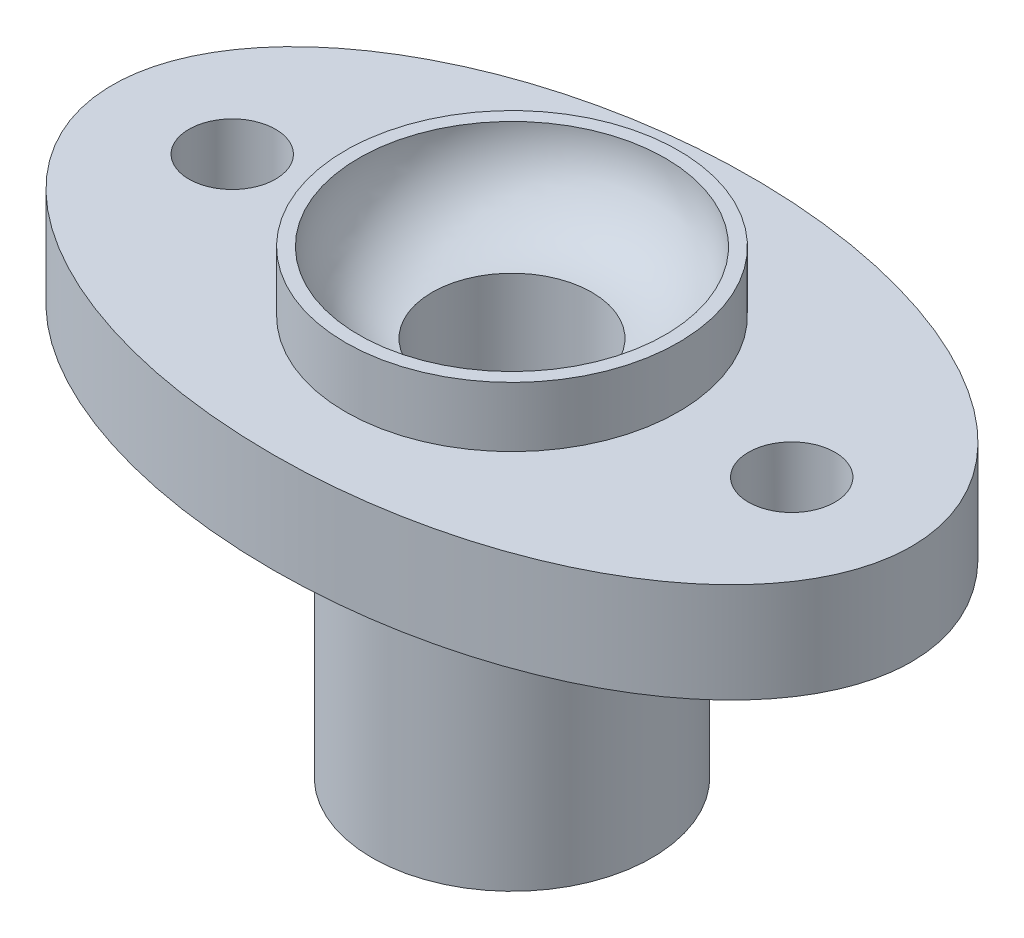
ISO-10303-21;
HEADER;
FILE_DESCRIPTION(('STEP AP214'),'2;1');
FILE_NAME('part.step','',(''),(''),'','','');
FILE_SCHEMA(('AUTOMOTIVE_DESIGN { 1 0 10303 214 1 1 1 1 }'));
ENDSEC;
DATA;
#1=APPLICATION_CONTEXT('core data for automotive mechanical design processes');
#2=APPLICATION_PROTOCOL_DEFINITION('international standard','automotive_design',2000,#1);
#3=PRODUCT_CONTEXT('',#1,'mechanical');
#4=PRODUCT('Part','Part','',(#3));
#5=PRODUCT_RELATED_PRODUCT_CATEGORY('part','',(#4));
#6=PRODUCT_DEFINITION_FORMATION('','',#4);
#7=PRODUCT_DEFINITION_CONTEXT('part definition',#1,'design');
#8=PRODUCT_DEFINITION('design','',#6,#7);
#9=PRODUCT_DEFINITION_SHAPE('','',#8);
#10=(LENGTH_UNIT() NAMED_UNIT(*) SI_UNIT(.MILLI.,.METRE.));
#11=(NAMED_UNIT(*) PLANE_ANGLE_UNIT() SI_UNIT($,.RADIAN.));
#12=(NAMED_UNIT(*) SI_UNIT($,.STERADIAN.) SOLID_ANGLE_UNIT());
#13=UNCERTAINTY_MEASURE_WITH_UNIT(LENGTH_MEASURE(1.E-05),#10,'distance_accuracy_value','');
#14=(GEOMETRIC_REPRESENTATION_CONTEXT(3) GLOBAL_UNCERTAINTY_ASSIGNED_CONTEXT((#13)) GLOBAL_UNIT_ASSIGNED_CONTEXT((#10,
#11,#12)) REPRESENTATION_CONTEXT('',''));
#15=CARTESIAN_POINT('',(0.,0.,0.));
#16=DIRECTION('',(0.,0.,1.));
#17=DIRECTION('',(1.,0.,0.));
#18=AXIS2_PLACEMENT_3D('',#15,#16,#17);
#19=CARTESIAN_POINT('',(0.,-33.9411254969543,0.));
#20=DIRECTION('',(0.,1.,0.));
#21=DIRECTION('',(0.,0.,1.));
#22=AXIS2_PLACEMENT_3D('',#19,#20,#21);
#23=CYLINDRICAL_SURFACE('',#22,12.);
#24=CARTESIAN_POINT('',(0.,2.41154273188011,0.));
#25=DIRECTION('',(0.,1.,0.));
#26=DIRECTION('',(0.,0.,1.));
#27=AXIS2_PLACEMENT_3D('',#24,#25,#26);
#28=CIRCLE('',#27,12.);
#29=CARTESIAN_POINT('',(0.,2.41154273188011,12.));
#30=VERTEX_POINT('',#29);
#31=EDGE_CURVE('E10',#30,#30,#28,.F.);
#32=ORIENTED_EDGE('',*,*,#31,.T.);
#33=EDGE_LOOP('',(#32));
#34=FACE_BOUND('',#33,.T.);
#35=CARTESIAN_POINT('',(0.,57.0417392568986,0.));
#36=DIRECTION('',(0.,1.,0.));
#37=DIRECTION('',(0.,0.,1.));
#38=AXIS2_PLACEMENT_3D('',#35,#36,#37);
#39=CIRCLE('',#38,12.);
#40=CARTESIAN_POINT('',(0.,57.0417392568986,12.));
#41=VERTEX_POINT('',#40);
#42=EDGE_CURVE('E63',#41,#41,#39,.F.);
#43=ORIENTED_EDGE('',*,*,#42,.F.);
#44=EDGE_LOOP('',(#43));
#45=FACE_BOUND('',#44,.T.);
#46=ADVANCED_FACE('F39',(#34,#45),#23,.F.);
#47=CARTESIAN_POINT('',(0.,45.,0.));
#48=DIRECTION('',(0.,-1.,0.));
#49=DIRECTION('',(0.,0.,-1.));
#50=AXIS2_PLACEMENT_3D('',#47,#48,#49);
#51=CYLINDRICAL_SURFACE('',#50,21.);
#52=CARTESIAN_POINT('',(0.,45.,0.));
#53=DIRECTION('',(0.,1.,0.));
#54=DIRECTION('',(0.,0.,1.));
#55=AXIS2_PLACEMENT_3D('',#52,#53,#54);
#56=CIRCLE('',#55,21.);
#57=CARTESIAN_POINT('',(0.,45.,-21.));
#58=VERTEX_POINT('',#57);
#59=EDGE_CURVE('E50',#58,#58,#56,.T.);
#60=CARTESIAN_POINT('',(0.,0.,0.));
#61=DIRECTION('',(0.,1.,0.));
#62=DIRECTION('',(0.,0.,1.));
#63=AXIS2_PLACEMENT_3D('',#60,#61,#62);
#64=CIRCLE('',#63,21.);
#65=CARTESIAN_POINT('',(0.,0.,-21.));
#66=VERTEX_POINT('',#65);
#67=EDGE_CURVE('E51',#66,#66,#64,.T.);
#68=CARTESIAN_POINT('',(0.,45.,-21.));
#69=CARTESIAN_POINT('',(0.,44.53125,-21.));
#70=CARTESIAN_POINT('',(0.,44.0625,-21.));
#71=CARTESIAN_POINT('',(0.,43.125,-21.));
#72=CARTESIAN_POINT('',(0.,42.65625,-21.));
#73=CARTESIAN_POINT('',(0.,41.71875,-21.));
#74=CARTESIAN_POINT('',(0.,41.25,-21.));
#75=CARTESIAN_POINT('',(0.,40.3125,-21.));
#76=CARTESIAN_POINT('',(0.,39.84375,-21.));
#77=CARTESIAN_POINT('',(0.,38.90625,-21.));
#78=CARTESIAN_POINT('',(0.,38.4375,-21.));
#79=CARTESIAN_POINT('',(0.,37.5,-21.));
#80=CARTESIAN_POINT('',(0.,37.03125,-21.));
#81=CARTESIAN_POINT('',(0.,36.09375,-21.));
#82=CARTESIAN_POINT('',(0.,35.625,-21.));
#83=CARTESIAN_POINT('',(0.,34.6875,-21.));
#84=CARTESIAN_POINT('',(0.,34.21875,-21.));
#85=CARTESIAN_POINT('',(0.,33.28125,-21.));
#86=CARTESIAN_POINT('',(0.,32.8125,-21.));
#87=CARTESIAN_POINT('',(0.,31.875,-21.));
#88=CARTESIAN_POINT('',(0.,31.40625,-21.));
#89=CARTESIAN_POINT('',(0.,30.46875,-21.));
#90=CARTESIAN_POINT('',(0.,30.,-21.));
#91=CARTESIAN_POINT('',(0.,29.0625,-21.));
#92=CARTESIAN_POINT('',(0.,28.59375,-21.));
#93=CARTESIAN_POINT('',(0.,27.65625,-21.));
#94=CARTESIAN_POINT('',(0.,27.1875,-21.));
#95=CARTESIAN_POINT('',(0.,26.25,-21.));
#96=CARTESIAN_POINT('',(0.,25.78125,-21.));
#97=CARTESIAN_POINT('',(0.,24.84375,-21.));
#98=CARTESIAN_POINT('',(0.,24.375,-21.));
#99=CARTESIAN_POINT('',(0.,23.4375,-21.));
#100=CARTESIAN_POINT('',(0.,22.96875,-21.));
#101=CARTESIAN_POINT('',(0.,22.03125,-21.));
#102=CARTESIAN_POINT('',(0.,21.5625,-21.));
#103=CARTESIAN_POINT('',(0.,20.625,-21.));
#104=CARTESIAN_POINT('',(0.,20.15625,-21.));
#105=CARTESIAN_POINT('',(0.,19.21875,-21.));
#106=CARTESIAN_POINT('',(0.,18.75,-21.));
#107=CARTESIAN_POINT('',(0.,17.8125,-21.));
#108=CARTESIAN_POINT('',(0.,17.34375,-21.));
#109=CARTESIAN_POINT('',(0.,16.40625,-21.));
#110=CARTESIAN_POINT('',(0.,15.9375,-21.));
#111=CARTESIAN_POINT('',(0.,15.,-21.));
#112=CARTESIAN_POINT('',(0.,14.53125,-21.));
#113=CARTESIAN_POINT('',(0.,13.59375,-21.));
#114=CARTESIAN_POINT('',(0.,13.125,-21.));
#115=CARTESIAN_POINT('',(0.,12.1875,-21.));
#116=CARTESIAN_POINT('',(0.,11.71875,-21.));
#117=CARTESIAN_POINT('',(0.,10.78125,-21.));
#118=CARTESIAN_POINT('',(0.,10.3125,-21.));
#119=CARTESIAN_POINT('',(0.,9.375,-21.));
#120=CARTESIAN_POINT('',(0.,8.90625,-21.));
#121=CARTESIAN_POINT('',(0.,7.96874999999999,-21.));
#122=CARTESIAN_POINT('',(0.,7.5,-21.));
#123=CARTESIAN_POINT('',(0.,6.5625,-21.));
#124=CARTESIAN_POINT('',(0.,6.09375,-21.));
#125=CARTESIAN_POINT('',(0.,5.15625,-21.));
#126=CARTESIAN_POINT('',(0.,4.68749999999999,-21.));
#127=CARTESIAN_POINT('',(0.,3.74999999999999,-21.));
#128=CARTESIAN_POINT('',(0.,3.28124999999999,-21.));
#129=CARTESIAN_POINT('',(0.,2.34374999999999,-21.));
#130=CARTESIAN_POINT('',(0.,1.87499999999999,-21.));
#131=CARTESIAN_POINT('',(0.,0.937499999999992,-21.));
#132=CARTESIAN_POINT('',(0.,0.468749999999993,-21.));
#133=CARTESIAN_POINT('',(0.,0.,-21.));
#134=B_SPLINE_CURVE_WITH_KNOTS('',3,(#68,#69,#70,#71,#72,#73,#74,#75,#76,#77,#78,#79,#80,#81,
#82,#83,#84,#85,#86,#87,#88,#89,#90,#91,#92,#93,#94,#95,#96,#97,#98,#99,#100,#101,#102,#103,
#104,#105,#106,#107,#108,#109,#110,#111,#112,#113,#114,#115,#116,#117,#118,#119,#120,#121,#122,
#123,#124,#125,#126,#127,#128,#129,#130,#131,#132,#133),.UNSPECIFIED.,.F.,.F.,(4,2,2,2,2,2,2,2,
2,2,2,2,2,2,2,2,2,2,2,2,2,2,2,2,2,2,2,2,2,2,2,2,4),(0.,1.40625,2.8125,4.21875000000001,
5.62500000000001,7.03125,8.4375,9.84375000000001,11.25,12.65625,14.0625,15.46875,16.875,
18.28125,19.6875,21.09375,22.5,23.90625,25.3125,26.71875,28.125,29.53125,30.9375,32.34375,33.75,
35.15625,36.5625,37.96875,39.375,40.78125,42.1875,43.59375,45.),.UNSPECIFIED.);
#135=EDGE_CURVE('BSEAM92',#58,#66,#134,.T.);
#136=ORIENTED_EDGE('',*,*,#59,.F.);
#137=ORIENTED_EDGE('',*,*,#67,.T.);
#138=ORIENTED_EDGE('',*,*,#135,.T.);
#139=ORIENTED_EDGE('',*,*,#135,.F.);
#140=EDGE_LOOP('',(#136,#138,#137,#139));
#141=FACE_BOUND('',#140,.T.);
#142=ADVANCED_FACE('F92',(#141),#51,.T.);
#143=CARTESIAN_POINT('',(0.,60.,0.));
#144=DIRECTION('',(0.,1.,0.));
#145=DIRECTION('',(1.,0.,0.));
#146=AXIS2_PLACEMENT_3D('',#143,#144,#145);
#147=ELLIPSE('',#146,60.,36.);
#148=DIRECTION('',(0.,-1.,0.));
#149=VECTOR('',#148,1.);
#150=SURFACE_OF_LINEAR_EXTRUSION('',#147,#149);
#151=CARTESIAN_POINT('',(60.,60.,0.));
#152=VERTEX_POINT('',#151);
#153=EDGE_CURVE('E57',#152,#152,#147,.T.);
#154=ORIENTED_EDGE('',*,*,#153,.F.);
#155=EDGE_LOOP('',(#154));
#156=FACE_BOUND('',#155,.T.);
#157=CARTESIAN_POINT('',(0.,45.,0.));
#158=DIRECTION('',(0.,1.,0.));
#159=DIRECTION('',(1.,0.,0.));
#160=AXIS2_PLACEMENT_3D('',#157,#158,#159);
#161=ELLIPSE('',#160,60.,36.);
#162=CARTESIAN_POINT('',(60.,45.,0.));
#163=VERTEX_POINT('',#162);
#164=EDGE_CURVE('E56',#163,#163,#161,.T.);
#165=ORIENTED_EDGE('',*,*,#164,.T.);
#166=EDGE_LOOP('',(#165));
#167=FACE_BOUND('',#166,.T.);
#168=ADVANCED_FACE('F93',(#156,#167),#150,.F.);
#169=CARTESIAN_POINT('',(0.,60.,0.));
#170=DIRECTION('',(0.,1.,0.));
#171=DIRECTION('',(0.,0.,1.));
#172=AXIS2_PLACEMENT_3D('',#169,#170,#171);
#173=PLANE('',#172);
#174=CARTESIAN_POINT('',(-42.,60.,0.));
#175=DIRECTION('',(0.,1.,0.));
#176=DIRECTION('',(0.,0.,1.));
#177=AXIS2_PLACEMENT_3D('',#174,#175,#176);
#178=CIRCLE('',#177,6.5);
#179=CARTESIAN_POINT('',(-42.,60.,6.5));
#180=VERTEX_POINT('',#179);
#181=EDGE_CURVE('E73',#180,#180,#178,.T.);
#182=ORIENTED_EDGE('',*,*,#181,.F.);
#183=EDGE_LOOP('',(#182));
#184=FACE_BOUND('',#183,.T.);
#185=CARTESIAN_POINT('',(42.,60.,0.));
#186=DIRECTION('',(0.,1.,0.));
#187=DIRECTION('',(0.,0.,-1.));
#188=AXIS2_PLACEMENT_3D('',#185,#186,#187);
#189=CIRCLE('',#188,6.5);
#190=CARTESIAN_POINT('',(42.,60.,-6.5));
#191=VERTEX_POINT('',#190);
#192=EDGE_CURVE('E61',#191,#191,#189,.T.);
#193=ORIENTED_EDGE('',*,*,#192,.F.);
#194=EDGE_LOOP('',(#193));
#195=FACE_BOUND('',#194,.T.);
#196=CARTESIAN_POINT('',(0.,60.,0.));
#197=DIRECTION('',(0.,1.,0.));
#198=DIRECTION('',(0.,0.,1.));
#199=AXIS2_PLACEMENT_3D('',#196,#197,#198);
#200=CIRCLE('',#199,25.);
#201=CARTESIAN_POINT('',(0.,60.,25.));
#202=VERTEX_POINT('',#201);
#203=EDGE_CURVE('E79',#202,#202,#200,.T.);
#204=ORIENTED_EDGE('',*,*,#203,.F.);
#205=EDGE_LOOP('',(#204));
#206=FACE_BOUND('',#205,.T.);
#207=ORIENTED_EDGE('',*,*,#153,.T.);
#208=EDGE_LOOP('',(#207));
#209=FACE_BOUND('',#208,.T.);
#210=ADVANCED_FACE('F94',(#184,#195,#206,#209),#173,.T.);
#211=CARTESIAN_POINT('',(0.,45.,0.));
#212=DIRECTION('',(0.,1.,0.));
#213=DIRECTION('',(0.,0.,1.));
#214=AXIS2_PLACEMENT_3D('',#211,#212,#213);
#215=PLANE('',#214);
#216=CARTESIAN_POINT('',(-42.,45.,0.));
#217=DIRECTION('',(0.,1.,0.));
#218=DIRECTION('',(0.,0.,1.));
#219=AXIS2_PLACEMENT_3D('',#216,#217,#218);
#220=CIRCLE('',#219,6.5);
#221=CARTESIAN_POINT('',(-42.,45.,6.5));
#222=VERTEX_POINT('',#221);
#223=EDGE_CURVE('E76',#222,#222,#220,.F.);
#224=ORIENTED_EDGE('',*,*,#223,.F.);
#225=EDGE_LOOP('',(#224));
#226=FACE_BOUND('',#225,.T.);
#227=CARTESIAN_POINT('',(42.,45.,0.));
#228=DIRECTION('',(0.,1.,0.));
#229=DIRECTION('',(0.,0.,1.));
#230=AXIS2_PLACEMENT_3D('',#227,#228,#229);
#231=CIRCLE('',#230,6.5);
#232=CARTESIAN_POINT('',(42.,45.,6.5));
#233=VERTEX_POINT('',#232);
#234=EDGE_CURVE('E70',#233,#233,#231,.F.);
#235=ORIENTED_EDGE('',*,*,#234,.F.);
#236=EDGE_LOOP('',(#235));
#237=FACE_BOUND('',#236,.T.);
#238=ORIENTED_EDGE('',*,*,#59,.T.);
#239=EDGE_LOOP('',(#238));
#240=FACE_BOUND('',#239,.T.);
#241=ORIENTED_EDGE('',*,*,#164,.F.);
#242=EDGE_LOOP('',(#241));
#243=FACE_BOUND('',#242,.T.);
#244=ADVANCED_FACE('F100',(#226,#237,#240,#243),#215,.F.);
#245=CARTESIAN_POINT('',(0.,69.,0.));
#246=DIRECTION('',(0.,-1.,0.));
#247=DIRECTION('',(0.,0.,-1.));
#248=AXIS2_PLACEMENT_3D('',#245,#246,#247);
#249=CYLINDRICAL_SURFACE('',#248,25.);
#250=CARTESIAN_POINT('',(0.,69.,0.));
#251=DIRECTION('',(0.,1.,0.));
#252=DIRECTION('',(0.,0.,1.));
#253=AXIS2_PLACEMENT_3D('',#250,#251,#252);
#254=CIRCLE('',#253,25.);
#255=CARTESIAN_POINT('',(0.,69.,25.));
#256=VERTEX_POINT('',#255);
#257=EDGE_CURVE('E81',#256,#256,#254,.T.);
#258=ORIENTED_EDGE('',*,*,#257,.F.);
#259=EDGE_LOOP('',(#258));
#260=FACE_BOUND('',#259,.T.);
#261=ORIENTED_EDGE('',*,*,#203,.T.);
#262=EDGE_LOOP('',(#261));
#263=FACE_BOUND('',#262,.T.);
#264=ADVANCED_FACE('F128',(#260,#263),#249,.T.);
#265=CARTESIAN_POINT('',(0.,69.,0.));
#266=DIRECTION('',(0.,1.,0.));
#267=DIRECTION('',(0.,0.,1.));
#268=AXIS2_PLACEMENT_3D('',#265,#266,#267);
#269=PLANE('',#268);
#270=CARTESIAN_POINT('',(0.,69.,0.));
#271=DIRECTION('',(0.,-1.,0.));
#272=DIRECTION('',(0.,0.,-1.));
#273=AXIS2_PLACEMENT_3D('',#270,#271,#272);
#274=CIRCLE('',#273,23.);
#275=CARTESIAN_POINT('',(0.,69.,-23.));
#276=VERTEX_POINT('',#275);
#277=EDGE_CURVE('E62',#276,#276,#274,.T.);
#278=ORIENTED_EDGE('',*,*,#277,.T.);
#279=EDGE_LOOP('',(#278));
#280=FACE_BOUND('',#279,.T.);
#281=ORIENTED_EDGE('',*,*,#257,.T.);
#282=EDGE_LOOP('',(#281));
#283=FACE_BOUND('',#282,.T.);
#284=ADVANCED_FACE('F127',(#280,#283),#269,.T.);
#285=CARTESIAN_POINT('',(42.,26.6152236891498,0.));
#286=DIRECTION('',(0.,1.,0.));
#287=DIRECTION('',(0.,0.,1.));
#288=AXIS2_PLACEMENT_3D('',#285,#286,#287);
#289=CYLINDRICAL_SURFACE('',#288,6.5);
#290=ORIENTED_EDGE('',*,*,#234,.T.);
#291=EDGE_LOOP('',(#290));
#292=FACE_BOUND('',#291,.T.);
#293=ORIENTED_EDGE('',*,*,#192,.T.);
#294=EDGE_LOOP('',(#293));
#295=FACE_BOUND('',#294,.T.);
#296=ADVANCED_FACE('F122',(#292,#295),#289,.F.);
#297=CARTESIAN_POINT('',(-42.,26.6152236891498,0.));
#298=DIRECTION('',(0.,1.,0.));
#299=DIRECTION('',(0.,0.,1.));
#300=AXIS2_PLACEMENT_3D('',#297,#298,#299);
#301=CYLINDRICAL_SURFACE('',#300,6.5);
#302=ORIENTED_EDGE('',*,*,#223,.T.);
#303=EDGE_LOOP('',(#302));
#304=FACE_BOUND('',#303,.T.);
#305=ORIENTED_EDGE('',*,*,#181,.T.);
#306=EDGE_LOOP('',(#305));
#307=FACE_BOUND('',#306,.T.);
#308=ADVANCED_FACE('F111',(#304,#307),#301,.F.);
#309=CARTESIAN_POINT('',(0.,69.,0.));
#310=DIRECTION('',(0.,-1.,0.));
#311=DIRECTION('',(0.,0.,-1.));
#312=AXIS2_PLACEMENT_3D('',#309,#310,#311);
#313=DEGENERATE_TOROIDAL_SURFACE('',#312,11.,12.,.T.);
#314=ORIENTED_EDGE('',*,*,#277,.F.);
#315=EDGE_LOOP('',(#314));
#316=FACE_BOUND('',#315,.T.);
#317=ORIENTED_EDGE('',*,*,#42,.T.);
#318=EDGE_LOOP('',(#317));
#319=FACE_BOUND('',#318,.T.);
#320=ADVANCED_FACE('F109',(#316,#319),#313,.F.);
#321=CARTESIAN_POINT('',(0.,2.41154273188011,0.));
#322=DIRECTION('',(0.,-1.,0.));
#323=DIRECTION('',(0.,0.,-1.));
#324=AXIS2_PLACEMENT_3D('',#321,#322,#323);
#325=CONICAL_SURFACE('',#324,12.,1.30899693899575);
#326=ORIENTED_EDGE('',*,*,#67,.F.);
#327=EDGE_LOOP('',(#326));
#328=FACE_BOUND('',#327,.T.);
#329=ORIENTED_EDGE('',*,*,#31,.F.);
#330=EDGE_LOOP('',(#329));
#331=FACE_BOUND('',#330,.T.);
#332=ADVANCED_FACE('F45',(#328,#331),#325,.F.);
#333=CLOSED_SHELL('',(#46,#142,#168,#210,#244,#264,#284,#296,#308,#320,#332));
#334=MANIFOLD_SOLID_BREP('B2',#333);
#335=ADVANCED_BREP_SHAPE_REPRESENTATION('',(#18,#334),#14);
#336=SHAPE_DEFINITION_REPRESENTATION(#9,#335);
ENDSEC;
END-ISO-10303-21;
